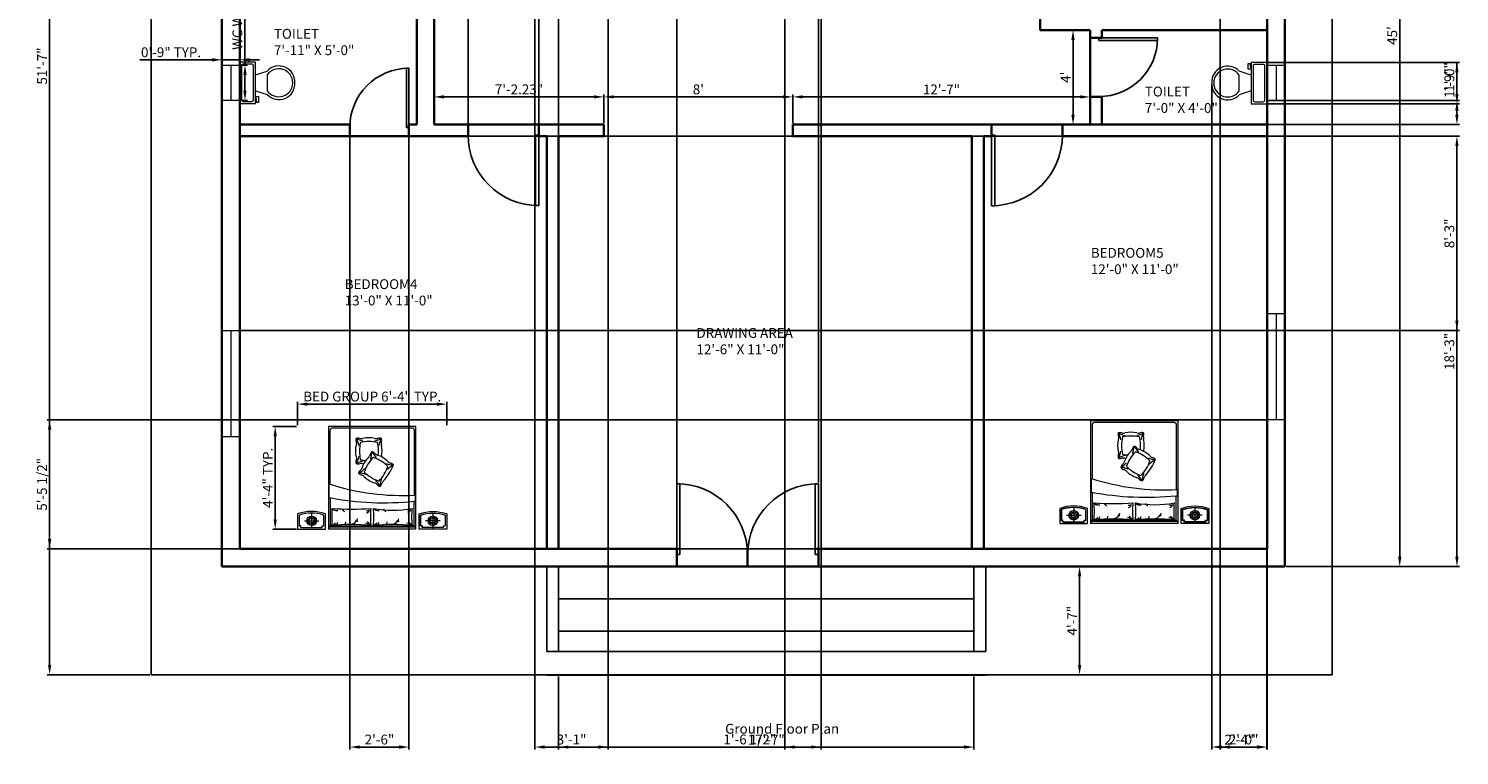
# Model space of a CAD drawing. Units: inches. Extents: x -938 to -211, y -366 to 366.
# Tile 1 of 4: x -938 to -211, y -366 to 4. Entities that reach past the tile are written whole.
import ezdxf

# ---------------------------------------------------------------- set-up
doc = ezdxf.new("R2010")
doc.units = ezdxf.units.IN
doc.header["$PDMODE"] = 35
doc.header["$PDSIZE"] = 5
for name, color, linetype, lineweight in [('A-ANNO-DIMS', 2, 'Continuous', 18), ('A-AREA-IDEN', 7, 'Continuous', 18), ('A-DOOR', 3, 'Continuous', 25), ('A-FLOR-FIXT', 9, 'Continuous', 18), ('A-FLOR-STRS', 7, 'Continuous', 25), ('A-GLAZ', 4, 'Continuous', 18), ('A-WALL', 7, 'Continuous', 35), ('C-PROP', 8, 'Continuous', 25), ('furn', 28, 'Continuous', 13), ('txt', 7, 'Continuous', 18)]:
    doc.layers.add(name, color=color, linetype=linetype, lineweight=lineweight)
doc.styles.get("Standard").update_dxf_attribs({"font": 'arial.ttf'})
doc.dimstyles.new('ISO-25', dxfattribs={"dimtxt": 5, "dimasz": 5, "dimexe": 1.25, "dimexo": 0.625, "dimtad": 1, "dimlunit": 3, "dimtxsty": 'Standard', "dimcen": 2.5, "dimadec": 0, "dimazin": 0, "dimtfac": 1, "dimtmove": 0, "dimatfit": 3, "dimfxl": 1, "dimarcsym": 0})

# ---------------------------------------------------------------- blocks, each defined once
blk = doc.blocks.new('*U2')
for p, q in [((0, 0), (0, -6)), ((40, 0), (40, -6))]:
    blk.add_line(p, q)
blk.add_lwpolyline([(0, 0), (0, 40), (1.75, 40), (1.75, 0)], close=True)
blk.add_arc((0, 0), 40, 0, 90)
blk = doc.blocks.new('*U4')
for p, q in [((9.5, -6), (9.5, -2)), ((-10, -8.5), (-8, -8.5)), ((-10, -9.5), (-10, -8.5)), ((-7, -9.5), (-10, -9.5)), ((-8, -8.5), (-8, -8)), ((-7, -8), (-7, -9.5)), ((-4, -8), (-6, -14)), ((4, -14), (-4, -14)), ((4, -8), (6, -14))]:
    blk.add_line(p, q)
blk.add_lwpolyline([(10.5, -8), (10.5, 0), (-10.5, 0), (-10.5, -8)], close=True)
for points in [[(-9.5, -2), (-9.5, -6)], [(8.5, -1), (-8.5, -1)], [(-8.5, -7), (8.5, -7)]]:
    blk.add_lwpolyline(points)
for centre, radius, start, end in [((-8.625, -1.875), 0.8839, 81.8699, 188.1301), ((-8.625, -6.125), 0.8839, 171.869898, 278.1301), ((8.625, -1.875), 0.8839, 351.8699, 98.1301), ((8.625, -6.125), 0.8839, 261.8699, 8.1301), ((-0.4772, -19.9188), 8.0953, 133.01722, 273.38), ((0.0374, -19.8731), 7.127, 124.50543, 269.7), ((-0.0373, -19.8731), 7.127, 270.3, 55.4946), ((0.4773, -19.9188), 8.0953, 266.62, 46.9828)]:
    blk.add_arc(centre, radius, start, end)
blk = doc.blocks.new('*D10')
at = {"layer": 'A-ANNO-DIMS', "color": 0, "lineweight": -2, "transparency": 16777216}
for p, q in [((-399.69, 2.79), (-408.98, 2.79)), ((-407.73, -2.21), (-407.73, -40.21)), ((-399.69, -45.21), (-408.98, -45.21))]:
    blk.add_line(p, q, dxfattribs=at)
at = {"layer": 'A-ANNO-DIMS', "color": 0, "transparency": 16777216}
for points in [[(-408.57, -2.21), (-406.9, -2.21), (-407.73, 2.79)], [(-408.57, -40.21), (-406.9, -40.21), (-407.73, -45.21)]]:
    blk.add_solid(points, dxfattribs=at)
at = {"layer": 'Defpoints', "color": 0, "transparency": 16777216}
for p in [(-399.06, 2.79), (-407.73, -45.21), (-399.06, -45.21)]:
    blk.add_point(p, dxfattribs=at)
at = {"layer": 'A-ANNO-DIMS', "color": 0, "transparency": 16777216, "insert": (-410.86, -21.21), "char_height": 5, "attachment_point": 5, "rotation": 90}
blk.add_mtext("4'", dxfattribs=at)
blk = doc.blocks.new('*D11')
at = {"layer": 'A-ANNO-DIMS', "color": 0, "lineweight": -2, "transparency": 16777216}
for p, q in [((-550.06, -44.58), (-550.06, -29.96)), ((-545.06, -31.21), (-404.06, -31.21)), ((-399.06, -44.58), (-399.06, -29.96))]:
    blk.add_line(p, q, dxfattribs=at)
at = {"layer": 'A-ANNO-DIMS', "color": 0, "transparency": 16777216}
for points in [[(-545.06, -30.38), (-545.06, -32.04), (-550.06, -31.21)], [(-404.06, -30.38), (-404.06, -32.04), (-399.06, -31.21)]]:
    blk.add_solid(points, dxfattribs=at)
at = {"layer": 'Defpoints', "color": 0, "transparency": 16777216}
for p in [(-399.06, -31.21), (-550.06, -45.21), (-399.06, -45.21)]:
    blk.add_point(p, dxfattribs=at)
at = {"layer": 'A-ANNO-DIMS', "color": 0, "transparency": 16777216, "insert": (-474.56, -28.07), "char_height": 5, "attachment_point": 5}
blk.add_mtext('12\'-7"', dxfattribs=at)
blk = doc.blocks.new('*D12')
at = {"layer": 'A-ANNO-DIMS', "color": 0, "lineweight": -2, "transparency": 16777216}
for p, q in [((-646.06, -44.58), (-646.06, -29.96)), ((-641.06, -31.21), (-555.06, -31.21)), ((-550.06, -44.58), (-550.06, -29.96))]:
    blk.add_line(p, q, dxfattribs=at)
at = {"layer": 'A-ANNO-DIMS', "color": 0, "transparency": 16777216}
for points in [[(-641.06, -30.38), (-641.06, -32.04), (-646.06, -31.21)], [(-555.06, -30.38), (-555.06, -32.04), (-550.06, -31.21)]]:
    blk.add_solid(points, dxfattribs=at)
at = {"layer": 'Defpoints', "color": 0, "transparency": 16777216}
for p in [(-550.06, -31.21), (-646.06, -45.21), (-550.06, -45.21)]:
    blk.add_point(p, dxfattribs=at)
at = {"layer": 'A-ANNO-DIMS', "color": 0, "transparency": 16777216, "insert": (-598.06, -28.03), "char_height": 5, "attachment_point": 5}
blk.add_mtext("8'", dxfattribs=at)
blk = doc.blocks.new('*D13')
at = {"layer": 'A-ANNO-DIMS', "color": 0, "lineweight": -2, "transparency": 16777216}
for p, q in [((-732.3, -44.58), (-732.3, -29.96)), ((-727.3, -31.21), (-651.06, -31.21)), ((-646.06, -44.58), (-646.06, -29.96))]:
    blk.add_line(p, q, dxfattribs=at)
at = {"layer": 'A-ANNO-DIMS', "color": 0, "transparency": 16777216}
for points in [[(-727.3, -30.38), (-727.3, -32.04), (-732.3, -31.21)], [(-651.06, -30.38), (-651.06, -32.04), (-646.06, -31.21)]]:
    blk.add_solid(points, dxfattribs=at)
at = {"layer": 'Defpoints', "color": 0, "transparency": 16777216}
for p in [(-646.06, -31.21), (-732.3, -45.21), (-646.06, -45.21)]:
    blk.add_point(p, dxfattribs=at)
at = {"layer": 'A-ANNO-DIMS', "color": 0, "transparency": 16777216, "insert": (-689.18, -28.03), "char_height": 5, "attachment_point": 5}
blk.add_mtext('7\'-2.23"', dxfattribs=at)
blk = doc.blocks.new('*D18')
at = {"layer": 'A-ANNO-DIMS', "color": 0, "lineweight": -2, "transparency": 16777216}
for p, q in [((-417.94, -270.02), (-403.15, -270.02)), ((-404.4, -275.02), (-404.4, -320.02)), ((-417.94, -325.02), (-403.15, -325.02))]:
    blk.add_line(p, q, dxfattribs=at)
at = {"layer": 'A-ANNO-DIMS', "color": 0, "transparency": 16777216}
for points in [[(-405.23, -275.02), (-403.57, -275.02), (-404.4, -270.02)], [(-405.23, -320.02), (-403.57, -320.02), (-404.4, -325.02)]]:
    blk.add_solid(points, dxfattribs=at)
at = {"layer": 'Defpoints', "color": 0, "transparency": 16777216}
for p in [(-418.56, -270.02), (-418.56, -325.02), (-404.4, -325.02)]:
    blk.add_point(p, dxfattribs=at)
at = {"layer": 'A-ANNO-DIMS', "color": 0, "transparency": 16777216, "insert": (-407.52, -297.52), "char_height": 5, "attachment_point": 5, "rotation": 90}
blk.add_mtext('4\'-7"', dxfattribs=at)
blk = doc.blocks.new('*D23')
at = {"layer": 'A-ANNO-DIMS', "color": 0, "lineweight": -2, "transparency": 16777216}
for p, q in [((-299.44, 269.98), (-240.52, 269.98)), ((-241.77, 264.98), (-241.77, -265.02)), ((-299.44, -270.02), (-240.52, -270.02))]:
    blk.add_line(p, q, dxfattribs=at)
at = {"layer": 'A-ANNO-DIMS', "color": 0, "transparency": 16777216}
for points in [[(-242.61, 264.98), (-240.94, 264.98), (-241.77, 269.98)], [(-242.61, -265.02), (-240.94, -265.02), (-241.77, -270.02)]]:
    blk.add_solid(points, dxfattribs=at)
at = {"layer": 'Defpoints', "color": 0, "transparency": 16777216}
for p in [(-300.06, 269.98), (-300.06, -270.02), (-241.77, -270.02)]:
    blk.add_point(p, dxfattribs=at)
at = {"layer": 'A-ANNO-DIMS', "color": 0, "transparency": 16777216, "insert": (-244.94, -0.02), "char_height": 5, "attachment_point": 5, "rotation": 90}
blk.add_mtext("45'", dxfattribs=at)
blk = doc.blocks.new('BED-DOUBLE-WITH-NIGHTSTANDS')
for p, q in [((-34.48, -4.26), (-27.06, -4.26)), ((-30.77, -7.97), (-30.77, -0.55)), ((-21.46, -1.59), (21.46, -1.59)), ((-21.24, -1.21), (-21.24, -14.04)), ((21.22, -1.21), (21.22, -15.71)), ((34.48, -4.26), (27.06, -4.26)), ((30.77, -7.97), (30.77, -0.55))]:
    blk.add_line(p, q)
for points in [[(-37.91, -7.71), (-37.91, 0), (-23.78, 0), (-23.78, -7.71, -0.181818)], [(-20.26, -10.53, 0.058596), (-20.26, -1.94, 0.036889), (-0.58, -1.94, 0.052163), (-0.58, -10.53, 0.093111)], [(0.7, -10.53, 0.058596), (0.7, -1.94, 0.036648), (20.51, -1.94, 0.052163), (20.51, -10.53, 0.036967)], [(37.91, -7.71), (37.91, 0), (23.78, 0), (23.78, -7.71, 0.181818)], [(-21.84, -14.04), (-21.24, -14.04, -0.072944), (21.82, -15.84), (21.82, -22.97, 0.092568), (-21.84, -17.31)]]:
    blk.add_lwpolyline(points, format="xyb", close=True)
for points in [[(-36.29, -0.77), (-36.29, -1.62), (-37.14, -1.62)], [(-36.22, -0.77), (-36.22, -1.7), (-37.14, -1.7)], [(-36.29, -0.77), (-25.39, -0.77)], [(-36.29, -0.85), (-25.39, -0.85)], [(-25.47, -0.77), (-25.47, -1.7), (-24.55, -1.7)], [(-25.39, -0.77), (-25.39, -1.62), (-24.55, -1.62)], [(-22.23, 0), (-22.23, -52.18), (22.23, -52.18), (22.23, 0)], [(21.82, 0), (21.82, -1.21), (-21.98, -1.21), (-21.98, 0), (22.23, 0)], [(25.39, -0.77), (25.39, -1.62), (24.55, -1.62)], [(25.47, -0.77), (25.47, -1.7), (24.55, -1.7)], [(36.29, -0.77), (25.39, -0.77)], [(36.29, -0.85), (25.39, -0.85)], [(36.22, -0.77), (36.22, -1.7), (37.14, -1.7)], [(36.29, -0.77), (36.29, -1.62), (37.14, -1.62)]]:
    blk.add_lwpolyline(points)
for points in [[(-24.55, -1.62), (-24.55, -7.18, -0.167087), (-37.14, -7.18), (-37.14, -1.62)], [(-24.62, -1.62), (-24.62, -7.12, -0.165559), (-37.06, -7.12), (-37.06, -1.62)], [(24.55, -1.62), (24.55, -7.17, 0.167087), (37.14, -7.17), (37.14, -1.62)], [(24.62, -1.62), (24.62, -7.12, 0.165559), (37.06, -7.12), (37.06, -1.62)], [(-21.46, -17.29), (-21.46, -50.12, 0.414214), (-20.18, -51.41), (20.18, -51.41, 0.414214), (21.46, -50.12), (21.46, -22.84)], [(-4.77, -25.48, 0.091296), (-3.99, -21.71, 0.091296), (-1.62, -24.74, 0.091296)], [(-7.96, -31.91, 0.111006), (-0.61, -36.48, 0.119549), (4.01, -29.05, 0.107813), (-3.31, -24.46)], [(-3.34, -24.47, 0.121865), (-7.96, -31.91, 0.121865)], [(0.12, -39.42, 0.159461), (1.12, -37.65, -0.076283), (1.91, -36.55, 0.115075), (5.13, -31.37, -0.076283), (5.77, -30.18, 0.159461), (6.92, -28.51)], [(3.15, -27.72, 0.091296), (6.92, -28.51, 0.091296), (3.88, -30.87, 0.091296)], [(-7.02, -33.41, 0.091296), (-10.79, -32.62, 0.091296), (-7.75, -30.26, 0.091296)], [(-2.67, -44.06, 0.111006), (5.98, -44.05, 0.119549), (5.98, -35.3, 0.033212), (3.32, -34.89)], [(0.9, -35.65, 0.091296), (0.12, -39.42, 0.091296), (-2.25, -36.39)], [(4.54, -34.62, 0.091296), (8.15, -33.3, 0.091296), (6.83, -36.91, 0.091296)], [(8.15, -46.15, 0.159461), (8.07, -44.13, -0.076283), (8.15, -42.78, 0.115075), (8.15, -36.68, -0.076283), (8.07, -35.33, 0.159461), (8.15, -33.3)], [(-1.08, -44.84, 0.091296), (-4.7, -46.15, 0.091296), (-3.37, -42.55, 0.091296)], [(6.83, -42.55, 0.091296), (8.15, -46.15, 0.091296), (4.54, -44.84)]]:
    blk.add_lwpolyline(points, format="xyb")
for centre, radius in [((-30.77, -4.26), 2.42), ((-30.77, -4.26), 1.31), ((30.77, -4.26), 2.42), ((30.77, -4.26), 1.31)]:
    blk.add_circle(centre, radius)
for centre, radius, start, end in [((-32.44, -3.65), 1.19, 232.30017, 292.53802), ((-32.43, -3.5), 1.56, 244.17003, 290.48975), ((-31.66, -2.67), 1.56, 208.17003, 254.48975), ((-31.77, -2.78), 1.19, 196.30017, 256.53802), ((-32.48, -4.75), 1.19, 268.30017, 328.53802), ((-32.56, -4.62), 1.56, 280.17003, 326.48975), ((-30.56, -2.45), 1.56, 172.17003, 218.48975), ((-30.71, -2.48), 1.19, 160.30017, 220.53802), ((-31.87, -5.66), 1.19, 304.30017, 4.53802), ((-29.53, -2.92), 1.56, 136.17003, 182.48975), ((-32.01, -5.6), 1.56, 316.17003, 2.48975), ((-29.67, -2.86), 1.19, 124.30017, 184.53802), ((-28.98, -3.9), 1.56, 100.17003, 146.48975), ((-29.06, -3.77), 1.19, 88.30017, 148.53802), ((-30.83, -6.04), 1.19, 340.30017, 40.53802), ((-30.99, -6.07), 1.56, 352.17003, 38.48975), ((-29.11, -5.02), 1.56, 64.17003, 110.48975), ((-29.1, -4.87), 1.19, 52.30017, 112.53802), ((-29.78, -5.74), 1.19, 16.30017, 76.53802), ((-29.88, -5.85), 1.56, 28.17003, 74.48975), ((-21.46, -0.82), 0.771, 180, 270), ((-15.69, 5.24), 8.51, 237.53791, 257.5233), ((-26.7, -9.98), 10.3, 36.49353, 51.27919), ((-15.35, -4.38), 2.13, 335.89274, 16.11919), ((-9.16, -7.04), 4.76, 96.68493, 148.3182), ((-4.35, -4.33), 3.34, 141.81741, 169.89867), ((-0.12, -4.8), 3.6, 130.53543, 160.35581), ((2.12, -7.83), 6.48, 114.64565, 134.15848), ((-5.74, -9.98), 10.3, 36.49353, 51.27919), ((5.27, 5.24), 8.51, 237.53791, 257.5233), ((5.61, -4.38), 2.13, 335.89274, 16.11919), ((11.8, -7.04), 4.76, 96.68493, 148.3182), ((16.61, -4.33), 3.34, 141.81741, 169.89867), ((20.84, -4.8), 3.6, 130.53543, 160.35581), ((23.08, -7.83), 6.48, 114.64565, 134.15848), ((21.46, -0.82), 0.771, 270, 0), ((29.1, -4.87), 1.19, 67.46198, 127.69983), ((29.11, -5.03), 1.56, 69.51025, 115.82997), ((29.88, -5.85), 1.56, 105.51025, 151.82997), ((29.78, -5.74), 1.19, 103.46198, 163.69983), ((29.06, -3.77), 1.19, 31.46198, 91.69983), ((28.98, -3.9), 1.56, 33.51025, 79.82997), ((30.99, -6.07), 1.56, 141.51025, 187.82997), ((30.83, -6.04), 1.19, 139.46198, 199.69983), ((29.67, -2.86), 1.19, 355.46198, 55.69983), ((32.01, -5.6), 1.56, 177.51025, 223.82997), ((29.53, -2.92), 1.56, 357.51025, 43.82997), ((31.87, -5.66), 1.19, 175.46198, 235.69983), ((32.56, -4.62), 1.56, 213.51025, 259.82997), ((32.48, -4.75), 1.19, 211.46198, 271.69983), ((30.71, -2.48), 1.19, 319.46198, 19.69983), ((30.73, -2.38), 1.56, 321.51025, 7.82997), ((32.61, -3.43), 1.56, 249.51025, 295.82997), ((32.62, -3.58), 1.19, 247.46198, 307.69983), ((31.94, -2.72), 1.19, 283.46198, 343.69983), ((31.84, -2.6), 1.56, 285.51025, 331.82997), ((-16.88, -10.73), 2.86, 114.2916, 160.9896), ((-18.36, -11.33), 1.95, 76.48229, 128.55627), ((-14.47, -16.51), 10.73, 36.20852, 45.08491), ((-6.53, -10.17), 0.72, 353.75428, 77.21866), ((-3.09, -12.99), 3.51, 44.40604, 96.83423), ((-2.43, -11.76), 2.23, 33.63488, 90.84559), ((4.08, -10.73), 2.86, 114.2916, 160.9896), ((2.6, -11.33), 1.95, 76.48229, 128.55627), ((6.49, -16.51), 10.73, 36.20852, 45.08491), ((14.43, -10.17), 0.72, 353.75428, 77.21866), ((17.87, -12.99), 3.51, 44.40604, 96.83423), ((18.53, -11.76), 2.23, 33.63488, 90.84559), ((-1.79, -24.12), 3.26, 132.46578, 168.70648), ((-4.85, -24.74), 3.14, 37.29372, 74.09733), ((15.27, -43.27), 28.15, 138.38179, 157.76439), ((-8.96, -21.45), 4.46, 315.58539, 333.03435), ((0.32, -19.25), 4.46, 233.29829, 250.74724), ((-5.44, -36.19), 13.43, 45.13065, 71.38844), ((7.15, -23.48), 4.46, 225.77185, 243.2208), ((4.59, -30.42), 3.01, 39.47264, 79.6505), ((-8.39, -30.41), 3.26, 222.65224, 258.89294), ((-11.03, -37.59), 4.46, 45.77185, 63.2208), ((1.56, -24.88), 13.43, 225.13065, 251.38844), ((1.73, -46.36), 13.43, 77.05756, 78.7033), ((5.69, -28.91), 4.46, 257.69876, 275.14771), ((7.19, -36.15), 3.01, 71.39955, 111.57741), ((8.38, -39.73), 13.43, 166.87111, 193.12889), ((-9.05, -43.74), 4.46, 355.03874, 12.4877), ((15.01, -39.64), 18.22, 173.19556, 194.02838), ((-4.2, -41.82), 4.46, 53.29829, 70.74724), ((1.37, -35.91), 3.73, 218.77541, 250.35713), ((-1.56, -45.28), 3.26, 159.36661, 195.60731), ((-3.83, -43.01), 3.26, 254.57915, 290.81985), ((-2.27, -50.5), 4.46, 77.69876, 95.14771), ((1.69, -33.06), 13.43, 257.05756, 283.31535), ((5.76, -50.48), 4.46, 85.2252, 102.67415), ((7.36, -42.51), 3.73, 250.70232, 282.28404)]:
    blk.add_arc(centre, radius, start, end)
blk = doc.blocks.new('WINDOW-54IN')
blk.add_line((54, 0), (0, 0))
blk.add_lwpolyline([(54, 4.5), (54, -4.5), (0, -4.5), (0, 4.5)], close=True)
blk = doc.blocks.new('WINDOW-18IN')
blk.add_line((18, 0), (0, 0))
blk.add_lwpolyline([(18, 4.5), (18, -4.5), (0, -4.5), (0, 4.5)], close=True)
blk = doc.blocks.new('*D29')
at = {"layer": 'A-ANNO-DIMS', "color": 0, "lineweight": -2, "transparency": 16777216}
for p, q in [((-801.65, -198.17), (-801.65, -186.17)), ((-730.82, -187.42), (-796.65, -187.42)), ((-725.82, -198.17), (-725.82, -186.17))]:
    blk.add_line(p, q, dxfattribs=at)
at = {"layer": 'A-ANNO-DIMS', "color": 0, "transparency": 16777216}
for points in [[(-796.65, -186.59), (-796.65, -188.25), (-801.65, -187.42)], [(-730.82, -186.59), (-730.82, -188.25), (-725.82, -187.42)]]:
    blk.add_solid(points, dxfattribs=at)
at = {"layer": 'Defpoints', "color": 0, "transparency": 16777216}
for p in [(-801.65, -187.42), (-801.65, -198.79), (-725.82, -198.79)]:
    blk.add_point(p, dxfattribs=at)
at = {"layer": 'A-ANNO-DIMS', "color": 0, "transparency": 16777216, "insert": (-763.73, -184.21), "char_height": 5, "attachment_point": 5}
blk.add_mtext('BED GROUP 6\'-4" TYP.', dxfattribs=at)
blk = doc.blocks.new('*D30')
at = {"layer": 'A-ANNO-DIMS', "color": 0, "lineweight": -2, "transparency": 16777216}
for p, q in [((-802.27, -198.79), (-814.27, -198.79)), ((-813.02, -203.79), (-813.02, -245.97)), ((-802.27, -250.97), (-814.27, -250.97))]:
    blk.add_line(p, q, dxfattribs=at)
at = {"layer": 'A-ANNO-DIMS', "color": 0, "transparency": 16777216}
for points in [[(-813.85, -203.79), (-812.19, -203.79), (-813.02, -198.79)], [(-813.85, -245.97), (-812.19, -245.97), (-813.02, -250.97)]]:
    blk.add_solid(points, dxfattribs=at)
at = {"layer": 'Defpoints', "color": 0, "transparency": 16777216}
for p in [(-801.65, -198.79), (-813.02, -250.97), (-801.65, -250.97)]:
    blk.add_point(p, dxfattribs=at)
at = {"layer": 'A-ANNO-DIMS', "color": 0, "transparency": 16777216, "insert": (-816.15, -224.88), "char_height": 5, "attachment_point": 5, "rotation": 90}
blk.add_mtext('4\'-4" TYP.', dxfattribs=at)
blk = doc.blocks.new('*D33')
at = {"layer": 'A-ANNO-DIMS', "color": 0, "lineweight": -2, "transparency": 16777216}
for p, q in [((-828.36, -15.05), (-828.36, 68.05)), ((-830.44, -15.05), (-827.11, -15.05)), ((-828.36, -28.05), (-828.36, -20.05)), ((-830.44, -33.05), (-827.11, -33.05))]:
    blk.add_line(p, q, dxfattribs=at)
at = {"layer": 'A-ANNO-DIMS', "color": 0, "transparency": 16777216}
for points in [[(-829.2, -20.05), (-827.53, -20.05), (-828.36, -15.05)], [(-829.2, -28.05), (-827.53, -28.05), (-828.36, -33.05)]]:
    blk.add_solid(points, dxfattribs=at)
at = {"layer": 'Defpoints', "color": 0, "transparency": 16777216}
for p in [(-831.06, -15.05), (-828.36, -15.05), (-831.06, -33.05)]:
    blk.add_point(p, dxfattribs=at)
at = {"layer": 'A-ANNO-DIMS', "color": 0, "transparency": 16777216, "insert": (-831.57, 29), "char_height": 5, "attachment_point": 5, "rotation": 90}
blk.add_mtext('WC WINDOW 1\'-6" TYP.', dxfattribs=at)
blk = doc.blocks.new('*D34')
at = {"layer": 'A-ANNO-DIMS', "color": 0, "lineweight": -2, "transparency": 16777216}
for p, q in [((-845.06, -12.35), (-881.79, -12.35)), ((-840.06, -14.42), (-840.06, -11.1)), ((-831.06, -12.35), (-840.06, -12.35)), ((-831.06, -14.42), (-831.06, -11.1)), ((-826.06, -12.35), (-821.06, -12.35))]:
    blk.add_line(p, q, dxfattribs=at)
at = {"layer": 'A-ANNO-DIMS', "color": 0, "transparency": 16777216}
for points in [[(-845.06, -11.52), (-845.06, -13.18), (-840.06, -12.35)], [(-826.06, -11.52), (-826.06, -13.18), (-831.06, -12.35)]]:
    blk.add_solid(points, dxfattribs=at)
at = {"layer": 'Defpoints', "color": 0, "transparency": 16777216}
for p in [(-840.06, -12.35), (-840.06, -15.05), (-831.06, -15.05)]:
    blk.add_point(p, dxfattribs=at)
at = {"layer": 'A-ANNO-DIMS', "color": 0, "transparency": 16777216, "insert": (-865.93, -9.17), "char_height": 5, "attachment_point": 5}
blk.add_mtext('0\'-9" TYP.', dxfattribs=at)
blk = doc.blocks.new('*D44')
at = {"layer": 'A-ANNO-DIMS', "color": 0, "lineweight": -2, "transparency": 16777216}
for p, q in [((-876.69, 293.98), (-928.86, 293.98)), ((-927.61, -320.02), (-927.61, 288.98)), ((-876.69, -325.02), (-928.86, -325.02))]:
    blk.add_line(p, q, dxfattribs=at)
at = {"layer": 'A-ANNO-DIMS', "color": 0, "transparency": 16777216}
for points in [[(-928.45, 288.98), (-926.78, 288.98), (-927.61, 293.98)], [(-928.45, -320.02), (-926.78, -320.02), (-927.61, -325.02)]]:
    blk.add_solid(points, dxfattribs=at)
at = {"layer": 'Defpoints', "color": 0, "transparency": 16777216}
for p in [(-927.61, 293.98), (-876.06, 293.98), (-876.06, -325.02)]:
    blk.add_point(p, dxfattribs=at)
at = {"layer": 'A-ANNO-DIMS', "color": 0, "transparency": 16777216, "insert": (-930.79, -15.52), "char_height": 5, "attachment_point": 5, "rotation": 90}
blk.add_mtext('51\'-7"', dxfattribs=at)
blk = doc.blocks.new('*D45')
at = {"layer": 'A-ANNO-DIMS', "color": 0, "lineweight": -2, "transparency": 16777216}
for p, q in [((-609.06, -227.28), (-609.06, 331.78)), ((-604.06, 330.53), (-542.06, 330.53)), ((-537.06, -227.28), (-537.06, 331.78))]:
    blk.add_line(p, q, dxfattribs=at)
at = {"layer": 'A-ANNO-DIMS', "color": 0, "transparency": 16777216}
for points in [[(-604.06, 331.37), (-604.06, 329.7), (-609.06, 330.53)], [(-542.06, 331.37), (-542.06, 329.7), (-537.06, 330.53)]]:
    blk.add_solid(points, dxfattribs=at)
at = {"layer": 'Defpoints', "color": 0, "transparency": 16777216}
for p in [(-537.06, 330.53), (-609.06, -227.9), (-537.06, -227.9)]:
    blk.add_point(p, dxfattribs=at)
at = {"layer": 'A-ANNO-DIMS', "color": 0, "transparency": 16777216, "insert": (-573.06, 333.71), "char_height": 5, "attachment_point": 5}
blk.add_mtext('6\'-0"', dxfattribs=at)
blk = doc.blocks.new('*D46')
at = {"layer": 'A-ANNO-DIMS', "color": 0, "lineweight": -2, "transparency": 16777216}
for p, q in [((-669.06, -325.84), (-669.06, -363.01)), ((-458.1, -325.84), (-458.1, -363.01)), ((-664.06, -361.76), (-463.1, -361.76))]:
    blk.add_line(p, q, dxfattribs=at)
at = {"layer": 'A-ANNO-DIMS', "color": 0, "transparency": 16777216}
for points in [[(-664.06, -360.93), (-664.06, -362.6), (-669.06, -361.76)], [(-463.1, -360.93), (-463.1, -362.6), (-458.1, -361.76)]]:
    blk.add_solid(points, dxfattribs=at)
at = {"layer": 'Defpoints', "color": 0, "transparency": 16777216}
for p in [(-669.06, -325.21), (-458.1, -325.21), (-458.1, -361.76)]:
    blk.add_point(p, dxfattribs=at)
at = {"layer": 'A-ANNO-DIMS', "color": 0, "transparency": 16777216, "insert": (-563.58, -358.63), "char_height": 5, "attachment_point": 5}
blk.add_mtext('17\'-7"', dxfattribs=at)
blk = doc.blocks.new('*D47')
at = {"layer": 'A-ANNO-DIMS', "color": 0, "lineweight": -2, "transparency": 16777216}
for p, q in [((-715.02, -44.58), (-715.02, 331.78)), ((-710.02, 330.53), (-684.06, 330.53)), ((-679.06, -44.58), (-679.06, 331.78))]:
    blk.add_line(p, q, dxfattribs=at)
at = {"layer": 'A-ANNO-DIMS', "color": 0, "transparency": 16777216}
for points in [[(-710.02, 331.37), (-710.02, 329.7), (-715.02, 330.53)], [(-684.06, 331.37), (-684.06, 329.7), (-679.06, 330.53)]]:
    blk.add_solid(points, dxfattribs=at)
at = {"layer": 'Defpoints', "color": 0, "transparency": 16777216}
for p in [(-679.06, 330.53), (-715.02, -45.21), (-679.06, -45.21)]:
    blk.add_point(p, dxfattribs=at)
at = {"layer": 'A-ANNO-DIMS', "color": 0, "transparency": 16777216, "insert": (-697.04, 333.71), "char_height": 5, "attachment_point": 5}
blk.add_mtext('3\'-0"', dxfattribs=at)
blk = doc.blocks.new('*D48')
at = {"layer": 'A-ANNO-DIMS', "color": 0, "lineweight": -2, "transparency": 16777216}
for p, q in [((-775.06, -45.83), (-775.06, -363.01)), ((-745.06, -45.83), (-745.06, -363.01)), ((-770.06, -361.76), (-750.06, -361.76))]:
    blk.add_line(p, q, dxfattribs=at)
at = {"layer": 'A-ANNO-DIMS', "color": 0, "transparency": 16777216}
for points in [[(-770.06, -360.93), (-770.06, -362.6), (-775.06, -361.76)], [(-750.06, -360.93), (-750.06, -362.6), (-745.06, -361.76)]]:
    blk.add_solid(points, dxfattribs=at)
at = {"layer": 'Defpoints', "color": 0, "transparency": 16777216}
for p in [(-775.06, -45.21), (-745.06, -45.21), (-745.06, -361.76)]:
    blk.add_point(p, dxfattribs=at)
at = {"layer": 'A-ANNO-DIMS', "color": 0, "transparency": 16777216, "insert": (-760.06, -358.59), "char_height": 5, "attachment_point": 5}
blk.add_mtext('2\'-6"', dxfattribs=at)
blk = doc.blocks.new('*D49')
at = {"layer": 'A-ANNO-DIMS', "color": 0, "lineweight": -2, "transparency": 16777216}
for p, q in [((-669.06, -260.39), (-669.06, 331.78)), ((-664.06, 330.53), (-614.06, 330.53)), ((-609.06, -260.39), (-609.06, 331.78))]:
    blk.add_line(p, q, dxfattribs=at)
at = {"layer": 'A-ANNO-DIMS', "color": 0, "transparency": 16777216}
for points in [[(-664.06, 331.37), (-664.06, 329.7), (-669.06, 330.53)], [(-614.06, 331.37), (-614.06, 329.7), (-609.06, 330.53)]]:
    blk.add_solid(points, dxfattribs=at)
at = {"layer": 'Defpoints', "color": 0, "transparency": 16777216}
for p in [(-609.06, 330.53), (-669.06, -261.02), (-609.06, -261.02)]:
    blk.add_point(p, dxfattribs=at)
at = {"layer": 'A-ANNO-DIMS', "color": 0, "transparency": 16777216, "insert": (-639.06, 333.71), "char_height": 5, "attachment_point": 5}
blk.add_mtext('5\'-0"', dxfattribs=at)
blk = doc.blocks.new('*D50')
at = {"layer": 'A-ANNO-DIMS', "color": 0, "lineweight": -2, "transparency": 16777216}
for p, q in [((-333.06, 98.36), (-333.06, -363.01)), ((-309.06, 98.36), (-309.06, -363.01)), ((-328.06, -361.76), (-314.06, -361.76))]:
    blk.add_line(p, q, dxfattribs=at)
at = {"layer": 'A-ANNO-DIMS', "color": 0, "transparency": 16777216}
for points in [[(-328.06, -360.93), (-328.06, -362.6), (-333.06, -361.76)], [(-314.06, -360.93), (-314.06, -362.6), (-309.06, -361.76)]]:
    blk.add_solid(points, dxfattribs=at)
at = {"layer": 'Defpoints', "color": 0, "transparency": 16777216}
for p in [(-333.06, 98.98), (-309.06, 98.98), (-309.06, -361.76)]:
    blk.add_point(p, dxfattribs=at)
at = {"layer": 'A-ANNO-DIMS', "color": 0, "transparency": 16777216, "insert": (-321.06, -358.59), "char_height": 5, "attachment_point": 5}
blk.add_mtext('2\'-0"', dxfattribs=at)
blk = doc.blocks.new('*D51')
at = {"layer": 'A-ANNO-DIMS', "color": 0, "lineweight": -2, "transparency": 16777216}
for p, q in [((-337.26, -24.79), (-337.26, -363.01)), ((-309.26, -35.29), (-309.26, -363.01)), ((-332.26, -361.76), (-314.26, -361.76))]:
    blk.add_line(p, q, dxfattribs=at)
at = {"layer": 'A-ANNO-DIMS', "color": 0, "transparency": 16777216}
for points in [[(-332.26, -360.93), (-332.26, -362.6), (-337.26, -361.76)], [(-314.26, -360.93), (-314.26, -362.6), (-309.26, -361.76)]]:
    blk.add_solid(points, dxfattribs=at)
at = {"layer": 'Defpoints', "color": 0, "transparency": 16777216}
for p in [(-337.26, -24.16), (-309.26, -34.66), (-309.26, -361.76)]:
    blk.add_point(p, dxfattribs=at)
at = {"layer": 'A-ANNO-DIMS', "color": 0, "transparency": 16777216, "insert": (-323.26, -358.63), "char_height": 5, "attachment_point": 5}
blk.add_mtext('2\'-4"', dxfattribs=at)
blk = doc.blocks.new('*D52')
at = {"layer": 'A-ANNO-DIMS', "color": 0, "lineweight": -2, "transparency": 16777216}
for p, q in [((-308.64, -13.66), (-211.46, -13.66)), ((-212.71, -18.66), (-212.71, -29.66)), ((-308.64, -34.66), (-211.46, -34.66))]:
    blk.add_line(p, q, dxfattribs=at)
at = {"layer": 'A-ANNO-DIMS', "color": 0, "transparency": 16777216}
for points in [[(-213.55, -18.66), (-211.88, -18.66), (-212.71, -13.66)], [(-213.55, -29.66), (-211.88, -29.66), (-212.71, -34.66)]]:
    blk.add_solid(points, dxfattribs=at)
at = {"layer": 'Defpoints', "color": 0, "transparency": 16777216}
for p in [(-309.26, -13.66), (-309.26, -34.66), (-212.71, -34.66)]:
    blk.add_point(p, dxfattribs=at)
at = {"layer": 'A-ANNO-DIMS', "color": 0, "transparency": 16777216, "insert": (-215.89, -24.16), "char_height": 5, "attachment_point": 5, "rotation": 90}
blk.add_mtext('1\'-9"', dxfattribs=at)
blk = doc.blocks.new('*D53')
at = {"layer": 'A-ANNO-DIMS', "color": 0, "lineweight": -2, "transparency": 16777216}
for p, q in [((-309.69, -195.37), (-928.86, -195.37)), ((-927.61, -256.02), (-927.61, -200.37)), ((-309.69, -261.02), (-928.86, -261.02))]:
    blk.add_line(p, q, dxfattribs=at)
at = {"layer": 'A-ANNO-DIMS', "color": 0, "transparency": 16777216}
for points in [[(-928.45, -200.37), (-926.78, -200.37), (-927.61, -195.37)], [(-928.45, -256.02), (-926.78, -256.02), (-927.61, -261.02)]]:
    blk.add_solid(points, dxfattribs=at)
at = {"layer": 'Defpoints', "color": 0, "transparency": 16777216}
for p in [(-927.61, -195.37), (-309.06, -195.37), (-309.06, -261.02)]:
    blk.add_point(p, dxfattribs=at)
at = {"layer": 'A-ANNO-DIMS', "color": 0, "transparency": 16777216, "insert": (-930.82, -228.19), "char_height": 5, "attachment_point": 5, "rotation": 90}
blk.add_mtext('5\'-5 1/2"', dxfattribs=at)
blk = doc.blocks.new('*D54')
at = {"layer": 'A-ANNO-DIMS', "color": 0, "lineweight": -2, "transparency": 16777216}
for p, q in [((-308.44, -51.21), (-211.46, -51.21)), ((-212.71, -265.02), (-212.71, -56.21)), ((-299.44, -270.02), (-211.46, -270.02))]:
    blk.add_line(p, q, dxfattribs=at)
at = {"layer": 'A-ANNO-DIMS', "color": 0, "transparency": 16777216}
for points in [[(-213.55, -56.21), (-211.88, -56.21), (-212.71, -51.21)], [(-213.55, -265.02), (-211.88, -265.02), (-212.71, -270.02)]]:
    blk.add_solid(points, dxfattribs=at)
at = {"layer": 'Defpoints', "color": 0, "transparency": 16777216}
for p in [(-309.06, -51.21), (-212.71, -51.21), (-300.06, -270.02)]:
    blk.add_point(p, dxfattribs=at)
at = {"layer": 'A-ANNO-DIMS', "color": 0, "transparency": 16777216, "insert": (-215.89, -160.61), "char_height": 5, "attachment_point": 5, "rotation": 90}
blk.add_mtext('18\'-3"', dxfattribs=at)
blk = doc.blocks.new('*D57')
at = {"layer": 'A-ANNO-DIMS', "color": 0, "lineweight": -2, "transparency": 16777216}
for p, q in [((-681.06, 260.36), (-681.06, -363.01)), ((-643.86, 260.36), (-643.86, -363.01)), ((-648.86, -361.76), (-676.06, -361.76))]:
    blk.add_line(p, q, dxfattribs=at)
at = {"layer": 'A-ANNO-DIMS', "color": 0, "transparency": 16777216}
for points in [[(-676.06, -360.93), (-676.06, -362.6), (-681.06, -361.76)], [(-648.86, -360.93), (-648.86, -362.6), (-643.86, -361.76)]]:
    blk.add_solid(points, dxfattribs=at)
at = {"layer": 'Defpoints', "color": 0, "transparency": 16777216}
for p in [(-681.06, 260.98), (-643.86, 260.98), (-681.06, -361.76)]:
    blk.add_point(p, dxfattribs=at)
at = {"layer": 'A-ANNO-DIMS', "color": 0, "transparency": 16777216, "insert": (-662.46, -358.58), "char_height": 5, "attachment_point": 5}
blk.add_mtext('3\'-1"', dxfattribs=at)
blk = doc.blocks.new('*D58')
at = {"layer": 'A-ANNO-DIMS', "color": 0, "lineweight": -2, "transparency": 16777216}
for p, q in [((-554.06, 260.36), (-554.06, -363.01)), ((-535.69, 260.36), (-535.69, -363.01)), ((-554.06, -361.76), (-584.78, -361.76)), ((-540.69, -361.76), (-549.06, -361.76))]:
    blk.add_line(p, q, dxfattribs=at)
at = {"layer": 'A-ANNO-DIMS', "color": 0, "transparency": 16777216}
for points in [[(-549.06, -360.93), (-549.06, -362.6), (-554.06, -361.76)], [(-540.69, -360.93), (-540.69, -362.6), (-535.69, -361.76)]]:
    blk.add_solid(points, dxfattribs=at)
at = {"layer": 'Defpoints', "color": 0, "transparency": 16777216}
for p in [(-554.06, 260.98), (-535.69, 260.98), (-554.06, -361.76)]:
    blk.add_point(p, dxfattribs=at)
at = {"layer": 'A-ANNO-DIMS', "color": 0, "transparency": 16777216, "insert": (-571.92, -358.55), "char_height": 5, "attachment_point": 5}
blk.add_mtext('1\'-6 1/2"', dxfattribs=at)
blk = doc.blocks.new('*D63')
at = {"layer": 'A-ANNO-DIMS', "color": 0, "lineweight": -2, "transparency": 16777216}
for p, q in [((-830.44, -51.21), (-211.46, -51.21)), ((-212.71, -56.21), (-212.71, -145.01)), ((-830.44, -150.01), (-211.46, -150.01))]:
    blk.add_line(p, q, dxfattribs=at)
at = {"layer": 'A-ANNO-DIMS', "color": 0, "transparency": 16777216}
for points in [[(-213.55, -56.21), (-211.88, -56.21), (-212.71, -51.21)], [(-213.55, -145.01), (-211.88, -145.01), (-212.71, -150.01)]]:
    blk.add_solid(points, dxfattribs=at)
at = {"layer": 'Defpoints', "color": 0, "transparency": 16777216}
for p in [(-831.06, -51.21), (-831.06, -150.01), (-212.71, -150.01)]:
    blk.add_point(p, dxfattribs=at)
at = {"layer": 'A-ANNO-DIMS', "color": 0, "transparency": 16777216, "insert": (-215.89, -100.61), "char_height": 5, "attachment_point": 5, "rotation": 90}
blk.add_mtext('8\'-3"', dxfattribs=at)
blk = doc.blocks.new('*D67')
at = {"layer": 'A-ANNO-DIMS', "color": 0, "lineweight": -2, "transparency": 16777216}
for p, q in [((-212.71, -33.13), (-212.71, -14.06)), ((-308.44, -33.13), (-211.46, -33.13)), ((-212.71, -40.21), (-212.71, -38.13)), ((-308.44, -45.21), (-211.46, -45.21))]:
    blk.add_line(p, q, dxfattribs=at)
at = {"layer": 'A-ANNO-DIMS', "color": 0, "transparency": 16777216}
for points in [[(-213.55, -38.13), (-211.88, -38.13), (-212.71, -33.13)], [(-213.55, -40.21), (-211.88, -40.21), (-212.71, -45.21)]]:
    blk.add_solid(points, dxfattribs=at)
at = {"layer": 'Defpoints', "color": 0, "transparency": 16777216}
for p in [(-309.06, -33.13), (-212.71, -33.13), (-309.06, -45.21)]:
    blk.add_point(p, dxfattribs=at)
at = {"layer": 'A-ANNO-DIMS', "color": 0, "transparency": 16777216, "insert": (-215.89, -21.09), "char_height": 5, "attachment_point": 5, "rotation": 90}
blk.add_mtext('1\'-0"', dxfattribs=at)

msp = doc.modelspace()

# ---------------------------------------------------------------- linework, layer by layer
at = {"layer": 'A-FLOR-STRS'}
for p, q in [((-675.062, -270.018), (-675.062, -313.105)), ((-669.062, -270.018), (-669.062, -313.105)), ((-458.1, -313.105), (-458.1, -270.018)), ((-452.1, -313.105), (-452.1, -270.018)), ((-458.1, -286.417), (-669.062, -286.417)), ((-458.1, -302.815), (-669.062, -302.815)), ((-675.062, -313.105), (-452.1, -313.105)), ((-675.062, -325.018), (-675.062, -325.213)), ((-675.062, -325.213), (-669.062, -325.213)), ((-669.062, -325.018), (-669.062, -325.213)), ((-669.062, -325.213), (-452.1, -325.213)), ((-458.1, -325.213), (-458.1, -325.018)), ((-452.1, -325.213), (-452.1, -325.018))]:
    msp.add_line(p, q, dxfattribs=at)
at = {"layer": 'A-WALL'}
for p, q in [((-300.062, 269.982), (-300.062, -270.018)), ((-309.062, 98.982), (-309.062, -51.209)), ((-424.341, 2.791), (-424.341, 55.343)), ((-840.062, -270.018), (-840.062, 14.791)), ((-831.062, -51.209), (-831.062, 14.791)), ((-741.062, 14.791), (-741.062, -45.209)), ((-732.296, 20.791), (-732.296, -45.209)), ((-412.577, 2.791), (-424.341, 2.791)), ((-399.062, 2.791), (-412.577, 2.791)), ((-399.062, -45.209), (-399.062, 2.791)), ((-393.062, 2.791), (-309.062, 2.791)), ((-393.062, -1.209), (-393.062, 2.791)), ((-393.062, -1.209), (-399.062, -1.209)), ((-393.062, -31.209), (-399.062, -31.209)), ((-393.062, -45.209), (-393.062, -31.209)), ((-775.062, -45.209), (-831.062, -45.209)), ((-775.062, -45.209), (-775.062, -51.209)), ((-741.062, -45.209), (-745.062, -45.209)), ((-745.062, -45.209), (-745.062, -51.209)), ((-732.296, -45.209), (-646.062, -45.209)), ((-715.062, -51.209), (-715.062, -45.209)), ((-679.062, -51.209), (-679.062, -45.209)), ((-646.062, -45.209), (-646.062, -51.209)), ((-550.062, -45.209), (-550.062, -51.209)), ((-550.062, -45.209), (-309.062, -45.209)), ((-449.062, -51.209), (-449.062, -45.209)), ((-413.062, -51.209), (-413.062, -45.209)), ((-831.062, -261.018), (-831.062, -51.209)), ((-741.062, -51.209), (-831.062, -51.209)), ((-741.062, -51.209), (-735.062, -51.209)), ((-735.062, -51.209), (-715.062, -51.209)), ((-679.062, -51.209), (-675.062, -51.209)), ((-675.062, -261.018), (-675.062, -51.209)), ((-669.062, -261.018), (-669.062, -51.209)), ((-669.062, -51.209), (-646.062, -51.209)), ((-550.062, -51.209), (-459.062, -51.209)), ((-459.062, -51.209), (-459.062, -261.018)), ((-453.062, -51.209), (-453.062, -261.018)), ((-453.062, -51.209), (-449.062, -51.209)), ((-413.062, -51.209), (-309.062, -51.209)), ((-309.062, -51.209), (-309.062, -261.018)), ((-607.49, -261.018), (-831.062, -261.018)), ((-609.062, -261.018), (-609.062, -270.018)), ((-572.898, -261.018), (-573.226, -261.018)), ((-573.062, -261.018), (-573.062, -270.018)), ((-309.062, -261.018), (-538.635, -261.018)), ((-537.062, -261.018), (-537.062, -270.018)), ((-609.062, -270.018), (-840.062, -270.018)), ((-609.062, -270.018), (-537.062, -270.018)), ((-300.062, -270.018), (-537.062, -270.018))]:
    msp.add_line(p, q, dxfattribs=at)
at = {"layer": 'C-PROP'}
for p, q in [((-276.062, 293.982), (-276.062, -325.018)), ((-876.062, 269.982), (-876.062, -325.018)), ((-300.062, -325.018), (-876.062, -325.018)), ((-300.062, -325.018), (-276.062, -325.018))]:
    msp.add_line(p, q, dxfattribs=at)

# ---------------------------------------------------------------- block references
at = {"layer": 'A-DOOR'}
for p, xscale, yscale, zscale, rotation in [((-394.587, -1.209), 0.7458564984336807, 0.7458564984336807, 0.7458564984336807, 269.9999999999999), ((-679.153, -50.589), 0.8967790055150446, 0.8967790055150446, 0.8967790055150446, 180), ((-449.062, -50.602), -0.898815867579402, 0.898815867579402, 0.898815867579402, 180)]:
    msp.add_blockref('*U2', p, dxfattribs=dict(at, xscale=xscale, yscale=yscale, zscale=zscale, rotation=rotation))
for p, xscale, yscale, zscale in [((-745.062, -46.699), -0.751649472173968, 0.751649472173968, 0.751649472173968), ((-609.062, -263.848), 0.8986880990233336, 0.8986880990233336, 0.8986880990233336), ((-537.062, -263.848), -0.8986880990233336, 0.8986880990233336, 0.8986880990233336)]:
    msp.add_blockref('*U2', p, dxfattribs=dict(at, xscale=xscale, yscale=yscale, zscale=zscale))
at = {"layer": 'A-FLOR-FIXT'}
for p, rotation in [((-831.062, -24.049), 90), ((-309.262, -24.164), 270)]:
    msp.add_blockref('*U4', p, dxfattribs=dict(at, rotation=rotation))
at = {"layer": 'A-GLAZ'}
for name, p, rotation in [('WINDOW-18IN', (-835.562, -33.05), 90.00000000000036), ('WINDOW-18IN', (-304.562, -33.127), 90.0000000000001), ('WINDOW-54IN', (-304.562, -195.37), 90.00000000000003), ('WINDOW-54IN', (-835.562, -204.011), 90.00000000000011)]:
    msp.add_blockref(name, p, dxfattribs=dict(at, rotation=rotation))
at = {"layer": 'furn', "rotation": 180}
for p in [(-376.602, -248.165), (-763.734, -250.972)]:
    msp.add_blockref('BED-DOUBLE-WITH-NIGHTSTANDS', p, dxfattribs=at)

# ---------------------------------------------------------------- texts
at = {"layer": 'A-AREA-IDEN', "char_height": 5, "attachment_point": 1}
for s, width, insert in [('TOILET\\P7\'-11" X 5\'-0"', 64.51229, (-813.69, 3.366)), ('TOILET\\P7\'-0" X 4\'-0"', 38.01699, (-371.256, -25.999)), ('BEDROOM5\\P12\'-0" X 11\'-0"', 100.3753, (-398.687, -108.003)), ('BEDROOM4\\P13\'-0" X 11\'-0"', 111.66682, (-777.704, -123.909)), ('DRAWING AREA\\P12\'-6" X 11\'-0"', 140.63534, (-599.012, -148.732))]:
    msp.add_mtext_dynamic_manual_height_columns(s, width=width, gutter_width=12.5, heights=[0], dxfattribs=dict(at, insert=insert))
at = {"layer": 'txt', "insert": (-584.466, -349.968), "char_height": 5, "attachment_point": 1}
msp.add_mtext_dynamic_manual_height_columns('Ground Floor Plan', width=296.69835, gutter_width=12.5, heights=[0], dxfattribs=at)

# ---------------------------------------------------------------- dimensions: what is measured, and where the dimension line sits
at = {"layer": 'A-ANNO-DIMS'}
for base, p1, p2, override, picture, middle in [((-679.062, 330.532), (-715.024, -45.209), (-679.062, -45.209), {"dimdec": 1, "dimlfac": 1, "dimrnd": 0, "dimzin": 1, "dimdsep": 46, "dimlunit": 4, "dimfrac": 2}, '*D47', (-697.043, 333.711)), ((-609.062, 330.532), (-669.062, -261.018), (-609.062, -261.018), {"dimdec": 1, "dimlfac": 1, "dimrnd": 0, "dimzin": 1, "dimdsep": 46, "dimlunit": 4, "dimfrac": 2}, '*D49', (-639.062, 333.71)), ((-537.062, 330.532), (-609.062, -227.9), (-537.062, -227.9), {"dimdec": 1, "dimlfac": 1, "dimrnd": 0, "dimzin": 1, "dimdsep": 46, "dimlunit": 4, "dimfrac": 2}, '*D45', (-573.062, 333.71)), ((-681.062, -361.763), (-643.859, 260.982), (-681.062, 260.982), {"dimdec": 1, "dimlfac": 1, "dimrnd": 0, "dimzin": 1, "dimdsep": 46, "dimlunit": 4, "dimfrac": 2}, '*D57', (-662.461, -358.584)), ((-554.062, -361.763), (-535.694, 260.982), (-554.062, 260.982), {"dimdec": 1, "dimlfac": 1, "dimrnd": 0, "dimzin": 1, "dimdsep": 46, "dimlunit": 4, "dimfrac": 2}, '*D58', (-571.923, -358.553)), ((-309.062, -361.763), (-333.062, 98.982), (-309.062, 98.982), {"dimdec": 1, "dimlfac": 1, "dimrnd": 0, "dimzin": 1, "dimdsep": 46, "dimlunit": 4, "dimfrac": 2}, '*D50', (-321.062, -358.586)), ((-646.062, -31.209), (-732.296, -45.209), (-646.062, -45.209), {"dimclrd": 0, "dimclre": 0, "dimclrt": 0}, '*D13', (-689.179, -28.029)), ((-550.062, -31.209), (-646.062, -45.209), (-550.062, -45.209), {"dimclrd": 0, "dimclre": 0, "dimclrt": 0}, '*D12', (-598.062, -28.031)), ((-399.062, -31.209), (-550.062, -45.209), (-399.062, -45.209), {"dimclrd": 0, "dimclre": 0, "dimclrt": 0}, '*D11', (-474.562, -28.074)), ((-309.262, -361.763), (-337.262, -24.164), (-309.262, -34.664), {"dimdec": 1, "dimlfac": 1, "dimrnd": 0, "dimzin": 1, "dimdsep": 46, "dimlunit": 4, "dimfrac": 2}, '*D51', (-323.262, -358.628)), ((-745.062, -361.763), (-775.062, -45.209), (-745.062, -45.209), {"dimdec": 1, "dimlfac": 1, "dimrnd": 0, "dimzin": 1, "dimdsep": 46, "dimlunit": 4, "dimfrac": 2}, '*D48', (-760.062, -358.586)), ((-458.1, -361.763), (-669.062, -325.213), (-458.1, -325.213), {"dimdec": 1, "dimlfac": 1, "dimrnd": 0, "dimzin": 1, "dimdsep": 46, "dimlunit": 4, "dimfrac": 2}, '*D46', (-563.581, -358.628))]:
    dim = msp.add_linear_dim(base=base, p1=p1, p2=p2, dimstyle='ISO-25', override=override, dxfattribs=at)
    dim.commit()
    dim.dimension.update_dxf_attribs({"geometry": picture, "text_midpoint": middle})
for base, p1, p2, override, picture, middle in [((-927.612, 293.982), (-876.062, -325.018), (-876.062, 293.982), {"dimdec": 1, "dimlfac": 1, "dimrnd": 0, "dimzin": 1, "dimdsep": 46, "dimlunit": 4, "dimfrac": 2}, '*D44', (-930.79, -15.518)), ((-241.773, -270.018), (-300.062, 269.982), (-300.062, -270.018), {"dimclrd": 0, "dimclre": 0, "dimclrt": 0}, '*D23', (-244.941, -0.018)), ((-407.733, -45.209), (-399.062, 2.791), (-399.062, -45.209), {"dimclrd": 0, "dimclre": 0, "dimclrt": 0}, '*D10', (-410.858, -21.209)), ((-212.712, -34.664), (-309.262, -13.664), (-309.262, -34.664), {"dimdec": 1, "dimlfac": 1, "dimrnd": 0, "dimzin": 1, "dimdsep": 46, "dimlunit": 4, "dimfrac": 2}, '*D52', (-215.89, -24.164)), ((-212.712, -33.127), (-309.062, -45.209), (-309.062, -33.127), {"dimdec": 1, "dimlfac": 1, "dimrnd": 0, "dimzin": 1, "dimdsep": 46, "dimlunit": 4, "dimfrac": 2}, '*D67', (-215.89, -21.091)), ((-212.712, -150.011), (-831.062, -51.209), (-831.062, -150.011), {"dimdec": 1, "dimlfac": 1, "dimrnd": 0, "dimzin": 1, "dimdsep": 46, "dimlunit": 4, "dimfrac": 2}, '*D63', (-215.891, -100.61)), ((-212.712, -51.209), (-300.062, -270.018), (-309.062, -51.209), {"dimdec": 1, "dimlfac": 1, "dimrnd": 0, "dimzin": 1, "dimdsep": 46, "dimlunit": 4, "dimfrac": 2}, '*D54', (-215.891, -160.613)), ((-927.612, -195.37), (-309.062, -261.018), (-309.062, -195.37), {"dimdec": 1, "dimlfac": 1, "dimrnd": 0, "dimzin": 1, "dimdsep": 46, "dimlunit": 4, "dimfrac": 2}, '*D53', (-930.823, -228.194)), ((-404.399, -325.018), (-418.562, -270.018), (-418.562, -325.018), {"dimclrd": 0, "dimclre": 0, "dimclrt": 0}, '*D18', (-407.524, -297.518))]:
    dim = msp.add_linear_dim(base=base, p1=p1, p2=p2, angle=90, dimstyle='ISO-25', override=override, dxfattribs=at)
    dim.commit()
    dim.dimension.update_dxf_attribs({"geometry": picture, "text_midpoint": middle})
for base, p1, p2, angle, text, picture, middle in [((-828.362, -15.049), (-831.062, -33.049), (-831.062, -15.049), 90, 'WC WINDOW <> TYP.', '*D33', (-831.574, 29)), ((-840.062, -12.349), (-831.062, -15.049), (-840.062, -15.049), 180, '<> TYP.', '*D34', (-865.926, -9.171)), ((-801.647, -187.421), (-725.822, -198.794), (-801.647, -198.794), 180, 'BED GROUP <> TYP.', '*D29', (-763.735, -184.209)), ((-813.021, -250.972), (-801.647, -198.794), (-801.647, -250.972), 270, '<> TYP.', '*D30', (-816.147, -224.883))]:
    dim = msp.add_linear_dim(base=base, p1=p1, p2=p2, angle=angle, text=text, dimstyle='ISO-25', override={"dimdec": 1, "dimlfac": 1, "dimrnd": 0, "dimzin": 1, "dimdsep": 46, "dimlunit": 4, "dimfrac": 2}, dxfattribs=at)
    dim.commit()
    dim.dimension.update_dxf_attribs({"geometry": picture, "text_midpoint": middle})

doc.saveas('drawing.dxf')
